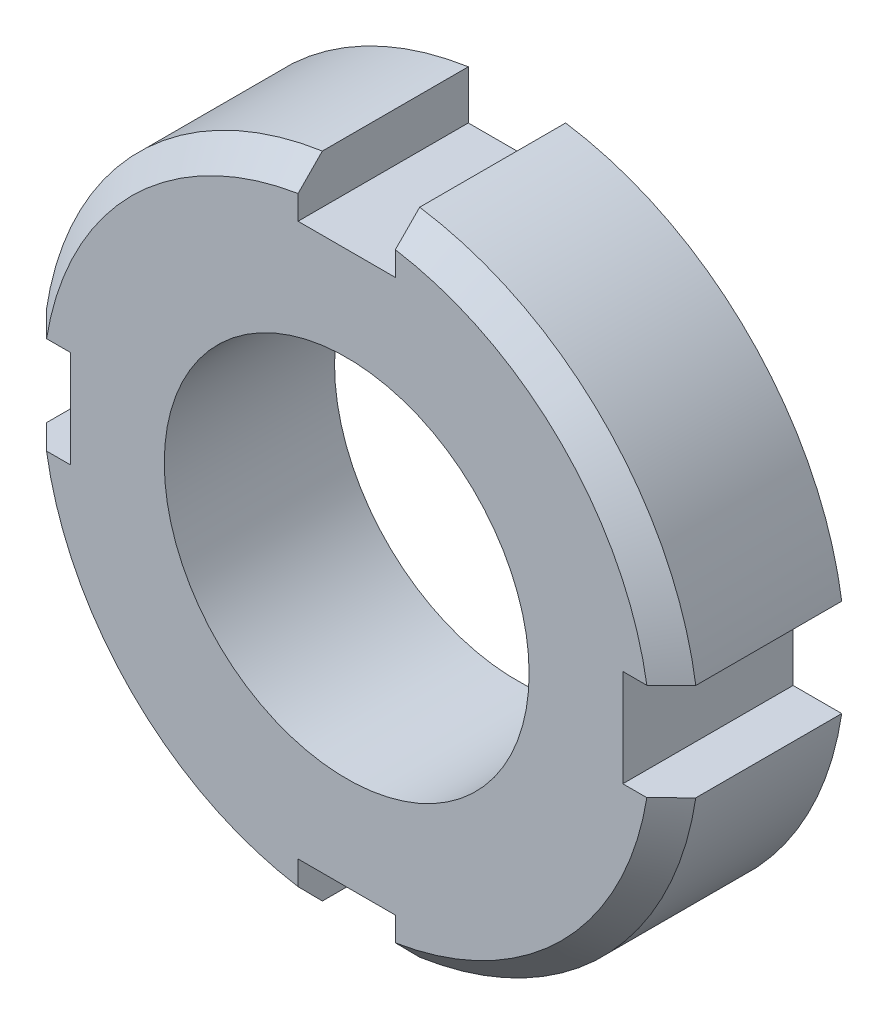
ISO-10303-21;
HEADER;
FILE_DESCRIPTION(('STEP AP214'),'2;1');
FILE_NAME('part.step','',(''),(''),'','','');
FILE_SCHEMA(('AUTOMOTIVE_DESIGN { 1 0 10303 214 1 1 1 1 }'));
ENDSEC;
DATA;
#1=APPLICATION_CONTEXT('core data for automotive mechanical design processes');
#2=APPLICATION_PROTOCOL_DEFINITION('international standard','automotive_design',2000,#1);
#3=PRODUCT_CONTEXT('',#1,'mechanical');
#4=PRODUCT('Part','Part','',(#3));
#5=PRODUCT_RELATED_PRODUCT_CATEGORY('part','',(#4));
#6=PRODUCT_DEFINITION_FORMATION('','',#4);
#7=PRODUCT_DEFINITION_CONTEXT('part definition',#1,'design');
#8=PRODUCT_DEFINITION('design','',#6,#7);
#9=PRODUCT_DEFINITION_SHAPE('','',#8);
#10=(LENGTH_UNIT() NAMED_UNIT(*) SI_UNIT(.MILLI.,.METRE.));
#11=(NAMED_UNIT(*) PLANE_ANGLE_UNIT() SI_UNIT($,.RADIAN.));
#12=(NAMED_UNIT(*) SI_UNIT($,.STERADIAN.) SOLID_ANGLE_UNIT());
#13=UNCERTAINTY_MEASURE_WITH_UNIT(LENGTH_MEASURE(1.E-05),#10,'distance_accuracy_value','');
#14=(GEOMETRIC_REPRESENTATION_CONTEXT(3) GLOBAL_UNCERTAINTY_ASSIGNED_CONTEXT((#13)) GLOBAL_UNIT_ASSIGNED_CONTEXT((#10,
#11,#12)) REPRESENTATION_CONTEXT('',''));
#15=CARTESIAN_POINT('',(0.,0.,0.));
#16=DIRECTION('',(0.,0.,1.));
#17=DIRECTION('',(1.,0.,0.));
#18=AXIS2_PLACEMENT_3D('',#15,#16,#17);
#19=CARTESIAN_POINT('',(-2.,11.3510299228187,3.5));
#20=DIRECTION('',(0.,-1.,0.));
#21=DIRECTION('',(0.,0.,-1.));
#22=AXIS2_PLACEMENT_3D('',#19,#20,#21);
#23=PLANE('',#22);
#24=DIRECTION('',(-1.,0.,0.));
#25=VECTOR('',#24,1.);
#26=CARTESIAN_POINT('',(-2.,11.3510299228187,-3.5));
#27=LINE('',#26,#25);
#28=CARTESIAN_POINT('',(2.,11.3510299228187,-3.5));
#29=VERTEX_POINT('',#28);
#30=CARTESIAN_POINT('',(-2.,11.3510299228187,-3.5));
#31=VERTEX_POINT('',#30);
#32=EDGE_CURVE('E211',#29,#31,#27,.T.);
#33=ORIENTED_EDGE('',*,*,#32,.T.);
#34=DIRECTION('',(0.,0.,-1.));
#35=VECTOR('',#34,1.);
#36=CARTESIAN_POINT('',(-2.,11.3510299228187,3.5));
#37=LINE('',#36,#35);
#38=CARTESIAN_POINT('',(-2.,11.3510299228187,3.5));
#39=VERTEX_POINT('',#38);
#40=EDGE_CURVE('E194',#39,#31,#37,.T.);
#41=ORIENTED_EDGE('',*,*,#40,.F.);
#42=DIRECTION('',(-1.,0.,0.));
#43=VECTOR('',#42,1.);
#44=CARTESIAN_POINT('',(-2.,11.3510299228187,3.5));
#45=LINE('',#44,#43);
#46=CARTESIAN_POINT('',(2.,11.3510299228187,3.5));
#47=VERTEX_POINT('',#46);
#48=EDGE_CURVE('E201',#47,#39,#45,.T.);
#49=ORIENTED_EDGE('',*,*,#48,.F.);
#50=DIRECTION('',(0.,0.,-1.));
#51=VECTOR('',#50,1.);
#52=CARTESIAN_POINT('',(2.,11.3510299228187,3.5));
#53=LINE('',#52,#51);
#54=EDGE_CURVE('E526',#47,#29,#53,.T.);
#55=ORIENTED_EDGE('',*,*,#54,.T.);
#56=EDGE_LOOP('',(#33,#41,#49,#55));
#57=FACE_BOUND('',#56,.T.);
#58=ADVANCED_FACE('F44',(#57),#23,.F.);
#59=CARTESIAN_POINT('',(-2.,11.3510299228187,3.5));
#60=DIRECTION('',(-1.,0.,0.));
#61=DIRECTION('',(0.,-1.,0.));
#62=AXIS2_PLACEMENT_3D('',#59,#60,#61);
#63=PLANE('',#62);
#64=DIRECTION('',(0.,0.,-1.));
#65=VECTOR('',#64,1.);
#66=CARTESIAN_POINT('',(-2.,13.3510299228187,3.5));
#67=LINE('',#66,#65);
#68=CARTESIAN_POINT('',(-2.,13.3510299228187,2.49999999999998));
#69=VERTEX_POINT('',#68);
#70=CARTESIAN_POINT('',(-2.,13.3510299228187,-3.5));
#71=VERTEX_POINT('',#70);
#72=EDGE_CURVE('E218',#69,#71,#67,.T.);
#73=ORIENTED_EDGE('',*,*,#72,.F.);
#74=CARTESIAN_POINT('',(-2.,13.3510299228187,2.49999999999998));
#75=CARTESIAN_POINT('',(-2.,13.1824298645057,2.66674542059407));
#76=CARTESIAN_POINT('',(-2.,13.0137908985623,2.83345146404985));
#77=CARTESIAN_POINT('',(-2.,12.6764351507074,3.16678479738352));
#78=CARTESIAN_POINT('',(-2.,12.5077183687956,3.33341208726107));
#79=CARTESIAN_POINT('',(-2.,12.3389626792531,3.5));
#80=B_SPLINE_CURVE_WITH_KNOTS('',3,(#74,#75,#76,#77,#78,#79),.UNSPECIFIED.,.F.,.F.,(4,2,4),(0.,
0.711386007616392,1.42277201821502),.UNSPECIFIED.);
#81=CARTESIAN_POINT('',(-2.,12.3389626792531,3.5));
#82=VERTEX_POINT('',#81);
#83=EDGE_CURVE('E198',#69,#82,#80,.T.);
#84=ORIENTED_EDGE('',*,*,#83,.T.);
#85=DIRECTION('',(0.,1.,0.));
#86=VECTOR('',#85,1.);
#87=CARTESIAN_POINT('',(-2.,11.3510299228187,3.5));
#88=LINE('',#87,#86);
#89=EDGE_CURVE('E190',#39,#82,#88,.T.);
#90=ORIENTED_EDGE('',*,*,#89,.F.);
#91=ORIENTED_EDGE('',*,*,#40,.T.);
#92=DIRECTION('',(0.,1.,0.));
#93=VECTOR('',#92,1.);
#94=CARTESIAN_POINT('',(-2.,11.3510299228187,-3.5));
#95=LINE('',#94,#93);
#96=EDGE_CURVE('E531',#31,#71,#95,.T.);
#97=ORIENTED_EDGE('',*,*,#96,.T.);
#98=EDGE_LOOP('',(#73,#84,#90,#91,#97));
#99=FACE_BOUND('',#98,.T.);
#100=ADVANCED_FACE('F188',(#99),#63,.F.);
#101=CARTESIAN_POINT('',(0.,0.,3.5));
#102=DIRECTION('',(0.,0.,-1.));
#103=DIRECTION('',(-1.,0.,0.));
#104=AXIS2_PLACEMENT_3D('',#101,#102,#103);
#105=CYLINDRICAL_SURFACE('',#104,13.5);
#106=DIRECTION('',(0.,0.,-1.));
#107=VECTOR('',#106,1.);
#108=CARTESIAN_POINT('',(-13.3510299228187,2.,3.5));
#109=LINE('',#108,#107);
#110=CARTESIAN_POINT('',(-13.3510299228187,2.,2.49999999999998));
#111=VERTEX_POINT('',#110);
#112=CARTESIAN_POINT('',(-13.3510299228187,2.,-3.5));
#113=VERTEX_POINT('',#112);
#114=EDGE_CURVE('E216',#111,#113,#109,.T.);
#115=ORIENTED_EDGE('',*,*,#114,.F.);
#116=CARTESIAN_POINT('',(0.,0.,2.49999999999998));
#117=DIRECTION('',(0.,0.,1.));
#118=DIRECTION('',(1.,0.,0.));
#119=AXIS2_PLACEMENT_3D('',#116,#117,#118);
#120=CIRCLE('',#119,13.5);
#121=EDGE_CURVE('E307',#111,#69,#120,.F.);
#122=ORIENTED_EDGE('',*,*,#121,.T.);
#123=ORIENTED_EDGE('',*,*,#72,.T.);
#124=CARTESIAN_POINT('',(0.,0.,-3.5));
#125=DIRECTION('',(0.,0.,1.));
#126=DIRECTION('',(1.,0.,0.));
#127=AXIS2_PLACEMENT_3D('',#124,#125,#126);
#128=CIRCLE('',#127,13.5);
#129=EDGE_CURVE('E537',#71,#113,#128,.T.);
#130=ORIENTED_EDGE('',*,*,#129,.T.);
#131=EDGE_LOOP('',(#115,#122,#123,#130));
#132=FACE_BOUND('',#131,.T.);
#133=ADVANCED_FACE('F319',(#132),#105,.T.);
#134=CARTESIAN_POINT('',(-11.3510299228187,2.,3.5));
#135=DIRECTION('',(0.,1.,0.));
#136=DIRECTION('',(-1.,0.,0.));
#137=AXIS2_PLACEMENT_3D('',#134,#135,#136);
#138=PLANE('',#137);
#139=DIRECTION('',(1.,0.,0.));
#140=VECTOR('',#139,1.);
#141=CARTESIAN_POINT('',(-11.3510299228187,2.,3.5));
#142=LINE('',#141,#140);
#143=CARTESIAN_POINT('',(-12.3389626792531,2.,3.5));
#144=VERTEX_POINT('',#143);
#145=CARTESIAN_POINT('',(-11.3510299228187,2.,3.5));
#146=VERTEX_POINT('',#145);
#147=EDGE_CURVE('E196',#144,#146,#142,.T.);
#148=ORIENTED_EDGE('',*,*,#147,.F.);
#149=CARTESIAN_POINT('',(-12.3389626792531,2.,3.5));
#150=CARTESIAN_POINT('',(-12.5077183687956,2.,3.33341208726107));
#151=CARTESIAN_POINT('',(-12.6764351507074,2.,3.16678479738352));
#152=CARTESIAN_POINT('',(-13.0137908985623,2.,2.83345146404985));
#153=CARTESIAN_POINT('',(-13.1824298645057,2.,2.66674542059407));
#154=CARTESIAN_POINT('',(-13.3510299228187,2.,2.49999999999998));
#155=B_SPLINE_CURVE_WITH_KNOTS('',3,(#149,#150,#151,#152,#153,#154),.UNSPECIFIED.,.F.,.F.,(4,2,
4),(0.,0.711386010598626,1.42277201821502),.UNSPECIFIED.);
#156=EDGE_CURVE('E303',#144,#111,#155,.T.);
#157=ORIENTED_EDGE('',*,*,#156,.T.);
#158=ORIENTED_EDGE('',*,*,#114,.T.);
#159=DIRECTION('',(1.,0.,0.));
#160=VECTOR('',#159,1.);
#161=CARTESIAN_POINT('',(-11.3510299228187,2.,-3.5));
#162=LINE('',#161,#160);
#163=CARTESIAN_POINT('',(-11.3510299228187,2.,-3.5));
#164=VERTEX_POINT('',#163);
#165=EDGE_CURVE('E536',#113,#164,#162,.T.);
#166=ORIENTED_EDGE('',*,*,#165,.T.);
#167=DIRECTION('',(0.,0.,-1.));
#168=VECTOR('',#167,1.);
#169=CARTESIAN_POINT('',(-11.3510299228187,2.,3.5));
#170=LINE('',#169,#168);
#171=EDGE_CURVE('E594',#146,#164,#170,.T.);
#172=ORIENTED_EDGE('',*,*,#171,.F.);
#173=EDGE_LOOP('',(#148,#157,#158,#166,#172));
#174=FACE_BOUND('',#173,.T.);
#175=ADVANCED_FACE('F313',(#174),#138,.F.);
#176=CARTESIAN_POINT('',(-11.3510299228187,-2.,3.5));
#177=DIRECTION('',(1.,0.,0.));
#178=DIRECTION('',(0.,0.,-1.));
#179=AXIS2_PLACEMENT_3D('',#176,#177,#178);
#180=PLANE('',#179);
#181=DIRECTION('',(0.,-1.,0.));
#182=VECTOR('',#181,1.);
#183=CARTESIAN_POINT('',(-11.3510299228187,-2.,-3.5));
#184=LINE('',#183,#182);
#185=CARTESIAN_POINT('',(-11.3510299228187,-2.,-3.5));
#186=VERTEX_POINT('',#185);
#187=EDGE_CURVE('E543',#164,#186,#184,.T.);
#188=ORIENTED_EDGE('',*,*,#187,.T.);
#189=DIRECTION('',(0.,0.,-1.));
#190=VECTOR('',#189,1.);
#191=CARTESIAN_POINT('',(-11.3510299228187,-2.,3.5));
#192=LINE('',#191,#190);
#193=CARTESIAN_POINT('',(-11.3510299228187,-2.,3.5));
#194=VERTEX_POINT('',#193);
#195=EDGE_CURVE('E595',#194,#186,#192,.T.);
#196=ORIENTED_EDGE('',*,*,#195,.F.);
#197=DIRECTION('',(0.,-1.,0.));
#198=VECTOR('',#197,1.);
#199=CARTESIAN_POINT('',(-11.3510299228187,-2.,3.5));
#200=LINE('',#199,#198);
#201=EDGE_CURVE('E618',#146,#194,#200,.T.);
#202=ORIENTED_EDGE('',*,*,#201,.F.);
#203=ORIENTED_EDGE('',*,*,#171,.T.);
#204=EDGE_LOOP('',(#188,#196,#202,#203));
#205=FACE_BOUND('',#204,.T.);
#206=ADVANCED_FACE('F295',(#205),#180,.F.);
#207=CARTESIAN_POINT('',(-11.3510299228187,-2.,3.5));
#208=DIRECTION('',(0.,-1.,0.));
#209=DIRECTION('',(1.,0.,0.));
#210=AXIS2_PLACEMENT_3D('',#207,#208,#209);
#211=PLANE('',#210);
#212=DIRECTION('',(0.,0.,-1.));
#213=VECTOR('',#212,1.);
#214=CARTESIAN_POINT('',(-13.3510299228187,-2.,3.5));
#215=LINE('',#214,#213);
#216=CARTESIAN_POINT('',(-13.3510299228187,-2.,2.5));
#217=VERTEX_POINT('',#216);
#218=CARTESIAN_POINT('',(-13.3510299228187,-2.,-3.5));
#219=VERTEX_POINT('',#218);
#220=EDGE_CURVE('E586',#217,#219,#215,.T.);
#221=ORIENTED_EDGE('',*,*,#220,.F.);
#222=CARTESIAN_POINT('',(-13.3510299228187,-2.,2.5));
#223=CARTESIAN_POINT('',(-13.1824298645057,-2.,2.66674542059408));
#224=CARTESIAN_POINT('',(-13.0137908985623,-2.,2.83345146404986));
#225=CARTESIAN_POINT('',(-12.6764351507074,-2.,3.16678479738353));
#226=CARTESIAN_POINT('',(-12.5077183687956,-2.,3.33341208726108));
#227=CARTESIAN_POINT('',(-12.3389626792531,-2.,3.5));
#228=B_SPLINE_CURVE_WITH_KNOTS('',3,(#222,#223,#224,#225,#226,#227),.UNSPECIFIED.,.F.,.F.,(4,2,
4),(0.,0.71138600761638,1.422772018215),.UNSPECIFIED.);
#229=CARTESIAN_POINT('',(-12.3389626792531,-2.,3.5));
#230=VERTEX_POINT('',#229);
#231=EDGE_CURVE('E300',#217,#230,#228,.T.);
#232=ORIENTED_EDGE('',*,*,#231,.T.);
#233=DIRECTION('',(-1.,0.,0.));
#234=VECTOR('',#233,1.);
#235=CARTESIAN_POINT('',(-11.3510299228187,-2.,3.5));
#236=LINE('',#235,#234);
#237=EDGE_CURVE('E615',#194,#230,#236,.T.);
#238=ORIENTED_EDGE('',*,*,#237,.F.);
#239=ORIENTED_EDGE('',*,*,#195,.T.);
#240=DIRECTION('',(-1.,0.,0.));
#241=VECTOR('',#240,1.);
#242=CARTESIAN_POINT('',(-11.3510299228187,-2.,-3.5));
#243=LINE('',#242,#241);
#244=EDGE_CURVE('E542',#186,#219,#243,.T.);
#245=ORIENTED_EDGE('',*,*,#244,.T.);
#246=EDGE_LOOP('',(#221,#232,#238,#239,#245));
#247=FACE_BOUND('',#246,.T.);
#248=ADVANCED_FACE('F288',(#247),#211,.F.);
#249=CARTESIAN_POINT('',(0.,0.,3.5));
#250=DIRECTION('',(0.,0.,-1.));
#251=DIRECTION('',(-1.,0.,0.));
#252=AXIS2_PLACEMENT_3D('',#249,#250,#251);
#253=CYLINDRICAL_SURFACE('',#252,13.5);
#254=DIRECTION('',(0.,0.,-1.));
#255=VECTOR('',#254,1.);
#256=CARTESIAN_POINT('',(-2.,-13.3510299228187,3.5));
#257=LINE('',#256,#255);
#258=CARTESIAN_POINT('',(-2.,-13.3510299228187,2.5));
#259=VERTEX_POINT('',#258);
#260=CARTESIAN_POINT('',(-2.,-13.3510299228187,-3.5));
#261=VERTEX_POINT('',#260);
#262=EDGE_CURVE('E587',#259,#261,#257,.T.);
#263=ORIENTED_EDGE('',*,*,#262,.F.);
#264=CARTESIAN_POINT('',(0.,0.,2.5));
#265=DIRECTION('',(0.,0.,1.));
#266=DIRECTION('',(1.,0.,0.));
#267=AXIS2_PLACEMENT_3D('',#264,#265,#266);
#268=CIRCLE('',#267,13.5);
#269=EDGE_CURVE('E277',#259,#217,#268,.F.);
#270=ORIENTED_EDGE('',*,*,#269,.T.);
#271=ORIENTED_EDGE('',*,*,#220,.T.);
#272=CARTESIAN_POINT('',(0.,0.,-3.5));
#273=DIRECTION('',(0.,0.,1.));
#274=DIRECTION('',(1.,0.,0.));
#275=AXIS2_PLACEMENT_3D('',#272,#273,#274);
#276=CIRCLE('',#275,13.5);
#277=EDGE_CURVE('E546',#219,#261,#276,.T.);
#278=ORIENTED_EDGE('',*,*,#277,.T.);
#279=EDGE_LOOP('',(#263,#270,#271,#278));
#280=FACE_BOUND('',#279,.T.);
#281=ADVANCED_FACE('F281',(#280),#253,.T.);
#282=CARTESIAN_POINT('',(-2.,-11.3510299228187,3.5));
#283=DIRECTION('',(-1.,0.,0.));
#284=DIRECTION('',(0.,-1.,0.));
#285=AXIS2_PLACEMENT_3D('',#282,#283,#284);
#286=PLANE('',#285);
#287=DIRECTION('',(0.,1.,0.));
#288=VECTOR('',#287,1.);
#289=CARTESIAN_POINT('',(-2.,-11.3510299228187,3.5));
#290=LINE('',#289,#288);
#291=CARTESIAN_POINT('',(-2.,-12.3389626792531,3.5));
#292=VERTEX_POINT('',#291);
#293=CARTESIAN_POINT('',(-2.,-11.3510299228187,3.5));
#294=VERTEX_POINT('',#293);
#295=EDGE_CURVE('E614',#292,#294,#290,.T.);
#296=ORIENTED_EDGE('',*,*,#295,.F.);
#297=CARTESIAN_POINT('',(-2.,-12.3389626792531,3.5));
#298=CARTESIAN_POINT('',(-2.,-12.5077183687956,3.33341208726108));
#299=CARTESIAN_POINT('',(-2.,-12.6764351507074,3.16678479738353));
#300=CARTESIAN_POINT('',(-2.,-13.0137908985623,2.83345146404986));
#301=CARTESIAN_POINT('',(-2.,-13.1824298645057,2.66674542059408));
#302=CARTESIAN_POINT('',(-2.,-13.3510299228187,2.5));
#303=B_SPLINE_CURVE_WITH_KNOTS('',3,(#297,#298,#299,#300,#301,#302),.UNSPECIFIED.,.F.,.F.,(4,2,
4),(0.,0.711386010598615,1.422772018215),.UNSPECIFIED.);
#304=EDGE_CURVE('E269',#292,#259,#303,.T.);
#305=ORIENTED_EDGE('',*,*,#304,.T.);
#306=ORIENTED_EDGE('',*,*,#262,.T.);
#307=DIRECTION('',(0.,1.,0.));
#308=VECTOR('',#307,1.);
#309=CARTESIAN_POINT('',(-2.,-11.3510299228187,-3.5));
#310=LINE('',#309,#308);
#311=CARTESIAN_POINT('',(-2.,-11.3510299228187,-3.5));
#312=VERTEX_POINT('',#311);
#313=EDGE_CURVE('E548',#261,#312,#310,.T.);
#314=ORIENTED_EDGE('',*,*,#313,.T.);
#315=DIRECTION('',(0.,0.,-1.));
#316=VECTOR('',#315,1.);
#317=CARTESIAN_POINT('',(-2.,-11.3510299228187,3.5));
#318=LINE('',#317,#316);
#319=EDGE_CURVE('E583',#294,#312,#318,.T.);
#320=ORIENTED_EDGE('',*,*,#319,.F.);
#321=EDGE_LOOP('',(#296,#305,#306,#314,#320));
#322=FACE_BOUND('',#321,.T.);
#323=ADVANCED_FACE('F283',(#322),#286,.F.);
#324=CARTESIAN_POINT('',(2.,-11.3510299228187,3.5));
#325=DIRECTION('',(0.,1.,0.));
#326=DIRECTION('',(0.,0.,1.));
#327=AXIS2_PLACEMENT_3D('',#324,#325,#326);
#328=PLANE('',#327);
#329=DIRECTION('',(1.,0.,0.));
#330=VECTOR('',#329,1.);
#331=CARTESIAN_POINT('',(2.,-11.3510299228187,-3.5));
#332=LINE('',#331,#330);
#333=CARTESIAN_POINT('',(2.,-11.3510299228187,-3.5));
#334=VERTEX_POINT('',#333);
#335=EDGE_CURVE('E553',#312,#334,#332,.T.);
#336=ORIENTED_EDGE('',*,*,#335,.T.);
#337=DIRECTION('',(0.,0.,-1.));
#338=VECTOR('',#337,1.);
#339=CARTESIAN_POINT('',(2.,-11.3510299228187,3.5));
#340=LINE('',#339,#338);
#341=CARTESIAN_POINT('',(2.,-11.3510299228187,3.5));
#342=VERTEX_POINT('',#341);
#343=EDGE_CURVE('E585',#342,#334,#340,.T.);
#344=ORIENTED_EDGE('',*,*,#343,.F.);
#345=DIRECTION('',(1.,0.,0.));
#346=VECTOR('',#345,1.);
#347=CARTESIAN_POINT('',(2.,-11.3510299228187,3.5));
#348=LINE('',#347,#346);
#349=EDGE_CURVE('E616',#294,#342,#348,.T.);
#350=ORIENTED_EDGE('',*,*,#349,.F.);
#351=ORIENTED_EDGE('',*,*,#319,.T.);
#352=EDGE_LOOP('',(#336,#344,#350,#351));
#353=FACE_BOUND('',#352,.T.);
#354=ADVANCED_FACE('F263',(#353),#328,.F.);
#355=CARTESIAN_POINT('',(2.,-11.3510299228187,3.5));
#356=DIRECTION('',(1.,0.,0.));
#357=DIRECTION('',(0.,1.,0.));
#358=AXIS2_PLACEMENT_3D('',#355,#356,#357);
#359=PLANE('',#358);
#360=DIRECTION('',(0.,0.,-1.));
#361=VECTOR('',#360,1.);
#362=CARTESIAN_POINT('',(2.,-13.3510299228187,3.5));
#363=LINE('',#362,#361);
#364=CARTESIAN_POINT('',(2.,-13.3510299228187,2.49999999999999));
#365=VERTEX_POINT('',#364);
#366=CARTESIAN_POINT('',(2.,-13.3510299228187,-3.5));
#367=VERTEX_POINT('',#366);
#368=EDGE_CURVE('E578',#365,#367,#363,.T.);
#369=ORIENTED_EDGE('',*,*,#368,.F.);
#370=CARTESIAN_POINT('',(2.,-13.3510299228187,2.49999999999999));
#371=CARTESIAN_POINT('',(2.,-13.1824298645057,2.66674542059407));
#372=CARTESIAN_POINT('',(2.,-13.0137908985623,2.83345146404985));
#373=CARTESIAN_POINT('',(2.,-12.6764351507074,3.16678479738352));
#374=CARTESIAN_POINT('',(2.,-12.5077183687956,3.33341208726107));
#375=CARTESIAN_POINT('',(2.,-12.3389626792531,3.5));
#376=B_SPLINE_CURVE_WITH_KNOTS('',3,(#370,#371,#372,#373,#374,#375),.UNSPECIFIED.,.F.,.F.,(4,2,
4),(0.,0.71138600761639,1.42277201821501),.UNSPECIFIED.);
#377=CARTESIAN_POINT('',(2.,-12.3389626792531,3.5));
#378=VERTEX_POINT('',#377);
#379=EDGE_CURVE('E265',#365,#378,#376,.T.);
#380=ORIENTED_EDGE('',*,*,#379,.T.);
#381=DIRECTION('',(0.,-1.,0.));
#382=VECTOR('',#381,1.);
#383=CARTESIAN_POINT('',(2.,-11.3510299228187,3.5));
#384=LINE('',#383,#382);
#385=EDGE_CURVE('E624',#342,#378,#384,.T.);
#386=ORIENTED_EDGE('',*,*,#385,.F.);
#387=ORIENTED_EDGE('',*,*,#343,.T.);
#388=DIRECTION('',(0.,-1.,0.));
#389=VECTOR('',#388,1.);
#390=CARTESIAN_POINT('',(2.,-11.3510299228187,-3.5));
#391=LINE('',#390,#389);
#392=EDGE_CURVE('E551',#334,#367,#391,.T.);
#393=ORIENTED_EDGE('',*,*,#392,.T.);
#394=EDGE_LOOP('',(#369,#380,#386,#387,#393));
#395=FACE_BOUND('',#394,.T.);
#396=ADVANCED_FACE('F257',(#395),#359,.F.);
#397=CARTESIAN_POINT('',(0.,0.,3.5));
#398=DIRECTION('',(0.,0.,-1.));
#399=DIRECTION('',(-1.,0.,0.));
#400=AXIS2_PLACEMENT_3D('',#397,#398,#399);
#401=CYLINDRICAL_SURFACE('',#400,13.5);
#402=DIRECTION('',(0.,0.,-1.));
#403=VECTOR('',#402,1.);
#404=CARTESIAN_POINT('',(13.3510299228187,-2.,3.5));
#405=LINE('',#404,#403);
#406=CARTESIAN_POINT('',(13.3510299228187,-2.,2.49999999999999));
#407=VERTEX_POINT('',#406);
#408=CARTESIAN_POINT('',(13.3510299228187,-2.,-3.5));
#409=VERTEX_POINT('',#408);
#410=EDGE_CURVE('E579',#407,#409,#405,.T.);
#411=ORIENTED_EDGE('',*,*,#410,.F.);
#412=CARTESIAN_POINT('',(0.,0.,2.49999999999999));
#413=DIRECTION('',(0.,0.,1.));
#414=DIRECTION('',(1.,0.,0.));
#415=AXIS2_PLACEMENT_3D('',#412,#413,#414);
#416=CIRCLE('',#415,13.5);
#417=EDGE_CURVE('E237',#407,#365,#416,.F.);
#418=ORIENTED_EDGE('',*,*,#417,.T.);
#419=ORIENTED_EDGE('',*,*,#368,.T.);
#420=CARTESIAN_POINT('',(0.,0.,-3.5));
#421=DIRECTION('',(0.,0.,1.));
#422=DIRECTION('',(1.,0.,0.));
#423=AXIS2_PLACEMENT_3D('',#420,#421,#422);
#424=CIRCLE('',#423,13.5);
#425=EDGE_CURVE('E558',#367,#409,#424,.T.);
#426=ORIENTED_EDGE('',*,*,#425,.T.);
#427=EDGE_LOOP('',(#411,#418,#419,#426));
#428=FACE_BOUND('',#427,.T.);
#429=ADVANCED_FACE('F255',(#428),#401,.T.);
#430=CARTESIAN_POINT('',(11.3510299228187,-2.,3.5));
#431=DIRECTION('',(0.,-1.,0.));
#432=DIRECTION('',(0.,0.,-1.));
#433=AXIS2_PLACEMENT_3D('',#430,#431,#432);
#434=PLANE('',#433);
#435=DIRECTION('',(-1.,0.,0.));
#436=VECTOR('',#435,1.);
#437=CARTESIAN_POINT('',(11.3510299228187,-2.,3.5));
#438=LINE('',#437,#436);
#439=CARTESIAN_POINT('',(12.3389626792531,-2.,3.5));
#440=VERTEX_POINT('',#439);
#441=CARTESIAN_POINT('',(11.3510299228187,-2.,3.5));
#442=VERTEX_POINT('',#441);
#443=EDGE_CURVE('E527',#440,#442,#438,.T.);
#444=ORIENTED_EDGE('',*,*,#443,.F.);
#445=CARTESIAN_POINT('',(12.3389626792531,-2.,3.5));
#446=CARTESIAN_POINT('',(12.5077183687956,-2.,3.33341208726107));
#447=CARTESIAN_POINT('',(12.6764351507074,-2.,3.16678479738352));
#448=CARTESIAN_POINT('',(13.0137908985623,-2.,2.83345146404985));
#449=CARTESIAN_POINT('',(13.1824298645057,-2.,2.66674542059407));
#450=CARTESIAN_POINT('',(13.3510299228187,-2.,2.49999999999999));
#451=B_SPLINE_CURVE_WITH_KNOTS('',3,(#445,#446,#447,#448,#449,#450),.UNSPECIFIED.,.F.,.F.,(4,2,
4),(0.,0.711386010598626,1.42277201821501),.UNSPECIFIED.);
#452=EDGE_CURVE('E233',#440,#407,#451,.T.);
#453=ORIENTED_EDGE('',*,*,#452,.T.);
#454=ORIENTED_EDGE('',*,*,#410,.T.);
#455=DIRECTION('',(-1.,0.,0.));
#456=VECTOR('',#455,1.);
#457=CARTESIAN_POINT('',(11.3510299228187,-2.,-3.5));
#458=LINE('',#457,#456);
#459=CARTESIAN_POINT('',(11.3510299228187,-2.,-3.5));
#460=VERTEX_POINT('',#459);
#461=EDGE_CURVE('E559',#409,#460,#458,.T.);
#462=ORIENTED_EDGE('',*,*,#461,.T.);
#463=DIRECTION('',(0.,0.,-1.));
#464=VECTOR('',#463,1.);
#465=CARTESIAN_POINT('',(11.3510299228187,-2.,3.5));
#466=LINE('',#465,#464);
#467=EDGE_CURVE('E574',#442,#460,#466,.T.);
#468=ORIENTED_EDGE('',*,*,#467,.F.);
#469=EDGE_LOOP('',(#444,#453,#454,#462,#468));
#470=FACE_BOUND('',#469,.T.);
#471=ADVANCED_FACE('F246',(#470),#434,.F.);
#472=CARTESIAN_POINT('',(11.3510299228187,2.,3.5));
#473=DIRECTION('',(-1.,0.,0.));
#474=DIRECTION('',(0.,0.,1.));
#475=AXIS2_PLACEMENT_3D('',#472,#473,#474);
#476=PLANE('',#475);
#477=DIRECTION('',(0.,1.,0.));
#478=VECTOR('',#477,1.);
#479=CARTESIAN_POINT('',(11.3510299228187,2.,-3.5));
#480=LINE('',#479,#478);
#481=CARTESIAN_POINT('',(11.3510299228187,2.,-3.5));
#482=VERTEX_POINT('',#481);
#483=EDGE_CURVE('E561',#460,#482,#480,.T.);
#484=ORIENTED_EDGE('',*,*,#483,.T.);
#485=DIRECTION('',(0.,0.,-1.));
#486=VECTOR('',#485,1.);
#487=CARTESIAN_POINT('',(11.3510299228187,2.,3.5));
#488=LINE('',#487,#486);
#489=CARTESIAN_POINT('',(11.3510299228187,2.,3.5));
#490=VERTEX_POINT('',#489);
#491=EDGE_CURVE('E572',#490,#482,#488,.T.);
#492=ORIENTED_EDGE('',*,*,#491,.F.);
#493=DIRECTION('',(0.,1.,0.));
#494=VECTOR('',#493,1.);
#495=CARTESIAN_POINT('',(11.3510299228187,2.,3.5));
#496=LINE('',#495,#494);
#497=EDGE_CURVE('E522',#442,#490,#496,.T.);
#498=ORIENTED_EDGE('',*,*,#497,.F.);
#499=ORIENTED_EDGE('',*,*,#467,.T.);
#500=EDGE_LOOP('',(#484,#492,#498,#499));
#501=FACE_BOUND('',#500,.T.);
#502=ADVANCED_FACE('F252',(#501),#476,.F.);
#503=CARTESIAN_POINT('',(11.3510299228187,2.,3.5));
#504=DIRECTION('',(0.,1.,0.));
#505=DIRECTION('',(0.,0.,1.));
#506=AXIS2_PLACEMENT_3D('',#503,#504,#505);
#507=PLANE('',#506);
#508=DIRECTION('',(0.,0.,-1.));
#509=VECTOR('',#508,1.);
#510=CARTESIAN_POINT('',(13.3510299228187,2.,3.5));
#511=LINE('',#510,#509);
#512=CARTESIAN_POINT('',(13.3510299228187,2.,2.49999999999998));
#513=VERTEX_POINT('',#512);
#514=CARTESIAN_POINT('',(13.3510299228187,2.,-3.5));
#515=VERTEX_POINT('',#514);
#516=EDGE_CURVE('E523',#513,#515,#511,.T.);
#517=ORIENTED_EDGE('',*,*,#516,.F.);
#518=CARTESIAN_POINT('',(13.3510299228187,2.,2.49999999999998));
#519=CARTESIAN_POINT('',(13.1824298645057,2.,2.66674542059407));
#520=CARTESIAN_POINT('',(13.0137908985623,2.,2.83345146404985));
#521=CARTESIAN_POINT('',(12.6764351507074,2.,3.16678479738352));
#522=CARTESIAN_POINT('',(12.5077183687956,2.,3.33341208726107));
#523=CARTESIAN_POINT('',(12.3389626792531,2.,3.5));
#524=B_SPLINE_CURVE_WITH_KNOTS('',3,(#518,#519,#520,#521,#522,#523),.UNSPECIFIED.,.F.,.F.,(4,2,
4),(0.,0.711386007616392,1.42277201821502),.UNSPECIFIED.);
#525=CARTESIAN_POINT('',(12.3389626792531,2.,3.5));
#526=VERTEX_POINT('',#525);
#527=EDGE_CURVE('E11',#513,#526,#524,.T.);
#528=ORIENTED_EDGE('',*,*,#527,.T.);
#529=DIRECTION('',(1.,0.,0.));
#530=VECTOR('',#529,1.);
#531=CARTESIAN_POINT('',(11.3510299228187,2.,3.5));
#532=LINE('',#531,#530);
#533=EDGE_CURVE('E516',#490,#526,#532,.T.);
#534=ORIENTED_EDGE('',*,*,#533,.F.);
#535=ORIENTED_EDGE('',*,*,#491,.T.);
#536=DIRECTION('',(1.,0.,0.));
#537=VECTOR('',#536,1.);
#538=CARTESIAN_POINT('',(11.3510299228187,2.,-3.5));
#539=LINE('',#538,#537);
#540=EDGE_CURVE('E563',#482,#515,#539,.T.);
#541=ORIENTED_EDGE('',*,*,#540,.T.);
#542=EDGE_LOOP('',(#517,#528,#534,#535,#541));
#543=FACE_BOUND('',#542,.T.);
#544=ADVANCED_FACE('F341',(#543),#507,.F.);
#545=CARTESIAN_POINT('',(0.,0.,3.5));
#546=DIRECTION('',(0.,0.,-1.));
#547=DIRECTION('',(-1.,0.,0.));
#548=AXIS2_PLACEMENT_3D('',#545,#546,#547);
#549=CYLINDRICAL_SURFACE('',#548,13.5);
#550=DIRECTION('',(0.,0.,-1.));
#551=VECTOR('',#550,1.);
#552=CARTESIAN_POINT('',(2.,13.3510299228187,3.5));
#553=LINE('',#552,#551);
#554=CARTESIAN_POINT('',(2.,13.3510299228187,2.49999999999998));
#555=VERTEX_POINT('',#554);
#556=CARTESIAN_POINT('',(2.,13.3510299228187,-3.5));
#557=VERTEX_POINT('',#556);
#558=EDGE_CURVE('E569',#555,#557,#553,.T.);
#559=ORIENTED_EDGE('',*,*,#558,.F.);
#560=CARTESIAN_POINT('',(0.,0.,2.49999999999998));
#561=DIRECTION('',(0.,0.,1.));
#562=DIRECTION('',(1.,0.,0.));
#563=AXIS2_PLACEMENT_3D('',#560,#561,#562);
#564=CIRCLE('',#563,13.5);
#565=EDGE_CURVE('E58',#555,#513,#564,.F.);
#566=ORIENTED_EDGE('',*,*,#565,.T.);
#567=ORIENTED_EDGE('',*,*,#516,.T.);
#568=CARTESIAN_POINT('',(0.,0.,-3.5));
#569=DIRECTION('',(0.,0.,1.));
#570=DIRECTION('',(1.,0.,0.));
#571=AXIS2_PLACEMENT_3D('',#568,#569,#570);
#572=CIRCLE('',#571,13.5);
#573=EDGE_CURVE('E564',#515,#557,#572,.T.);
#574=ORIENTED_EDGE('',*,*,#573,.T.);
#575=EDGE_LOOP('',(#559,#566,#567,#574));
#576=FACE_BOUND('',#575,.T.);
#577=ADVANCED_FACE('F338',(#576),#549,.T.);
#578=CARTESIAN_POINT('',(2.,11.3510299228187,3.5));
#579=DIRECTION('',(1.,0.,0.));
#580=DIRECTION('',(0.,1.,0.));
#581=AXIS2_PLACEMENT_3D('',#578,#579,#580);
#582=PLANE('',#581);
#583=DIRECTION('',(0.,-1.,0.));
#584=VECTOR('',#583,1.);
#585=CARTESIAN_POINT('',(2.,11.3510299228187,3.5));
#586=LINE('',#585,#584);
#587=CARTESIAN_POINT('',(2.,12.3389626792531,3.5));
#588=VERTEX_POINT('',#587);
#589=EDGE_CURVE('E210',#588,#47,#586,.T.);
#590=ORIENTED_EDGE('',*,*,#589,.F.);
#591=CARTESIAN_POINT('',(2.,12.3389626792531,3.5));
#592=CARTESIAN_POINT('',(2.,12.5077183687956,3.33341208726107));
#593=CARTESIAN_POINT('',(2.,12.6764351507074,3.16678479738352));
#594=CARTESIAN_POINT('',(2.,13.0137908985623,2.83345146404985));
#595=CARTESIAN_POINT('',(2.,13.1824298645057,2.66674542059407));
#596=CARTESIAN_POINT('',(2.,13.3510299228187,2.49999999999998));
#597=B_SPLINE_CURVE_WITH_KNOTS('',3,(#591,#592,#593,#594,#595,#596),.UNSPECIFIED.,.F.,.F.,(4,2,
4),(0.,0.711386010598626,1.42277201821502),.UNSPECIFIED.);
#598=EDGE_CURVE('E73',#588,#555,#597,.T.);
#599=ORIENTED_EDGE('',*,*,#598,.T.);
#600=ORIENTED_EDGE('',*,*,#558,.T.);
#601=DIRECTION('',(0.,-1.,0.));
#602=VECTOR('',#601,1.);
#603=CARTESIAN_POINT('',(2.,11.3510299228187,-3.5));
#604=LINE('',#603,#602);
#605=EDGE_CURVE('E212',#557,#29,#604,.T.);
#606=ORIENTED_EDGE('',*,*,#605,.T.);
#607=ORIENTED_EDGE('',*,*,#54,.F.);
#608=EDGE_LOOP('',(#590,#599,#600,#606,#607));
#609=FACE_BOUND('',#608,.T.);
#610=ADVANCED_FACE('F334',(#609),#582,.F.);
#611=CARTESIAN_POINT('',(0.,0.,3.5));
#612=DIRECTION('',(0.,0.,1.));
#613=DIRECTION('',(1.,0.,0.));
#614=AXIS2_PLACEMENT_3D('',#611,#612,#613);
#615=PLANE('',#614);
#616=CARTESIAN_POINT('',(0.,0.,3.5));
#617=DIRECTION('',(0.,0.,1.));
#618=DIRECTION('',(1.,0.,0.));
#619=AXIS2_PLACEMENT_3D('',#616,#617,#618);
#620=CIRCLE('',#619,7.5);
#621=CARTESIAN_POINT('',(7.5,0.,3.5));
#622=VERTEX_POINT('',#621);
#623=EDGE_CURVE('E632',#622,#622,#620,.T.);
#624=ORIENTED_EDGE('',*,*,#623,.F.);
#625=EDGE_LOOP('',(#624));
#626=FACE_BOUND('',#625,.T.);
#627=ORIENTED_EDGE('',*,*,#385,.T.);
#628=CARTESIAN_POINT('',(0.,0.,3.5));
#629=DIRECTION('',(0.,0.,1.));
#630=DIRECTION('',(1.,0.,0.));
#631=AXIS2_PLACEMENT_3D('',#628,#629,#630);
#632=CIRCLE('',#631,12.5);
#633=EDGE_CURVE('E226',#378,#440,#632,.T.);
#634=ORIENTED_EDGE('',*,*,#633,.T.);
#635=ORIENTED_EDGE('',*,*,#443,.T.);
#636=ORIENTED_EDGE('',*,*,#497,.T.);
#637=ORIENTED_EDGE('',*,*,#533,.T.);
#638=CARTESIAN_POINT('',(0.,0.,3.5));
#639=DIRECTION('',(0.,0.,1.));
#640=DIRECTION('',(1.,0.,0.));
#641=AXIS2_PLACEMENT_3D('',#638,#639,#640);
#642=CIRCLE('',#641,12.5);
#643=EDGE_CURVE('E213',#526,#588,#642,.T.);
#644=ORIENTED_EDGE('',*,*,#643,.T.);
#645=ORIENTED_EDGE('',*,*,#589,.T.);
#646=ORIENTED_EDGE('',*,*,#48,.T.);
#647=ORIENTED_EDGE('',*,*,#89,.T.);
#648=CARTESIAN_POINT('',(0.,0.,3.5));
#649=DIRECTION('',(0.,0.,1.));
#650=DIRECTION('',(1.,0.,0.));
#651=AXIS2_PLACEMENT_3D('',#648,#649,#650);
#652=CIRCLE('',#651,12.5);
#653=EDGE_CURVE('E217',#82,#144,#652,.T.);
#654=ORIENTED_EDGE('',*,*,#653,.T.);
#655=ORIENTED_EDGE('',*,*,#147,.T.);
#656=ORIENTED_EDGE('',*,*,#201,.T.);
#657=ORIENTED_EDGE('',*,*,#237,.T.);
#658=CARTESIAN_POINT('',(0.,0.,3.5));
#659=DIRECTION('',(0.,0.,1.));
#660=DIRECTION('',(1.,0.,0.));
#661=AXIS2_PLACEMENT_3D('',#658,#659,#660);
#662=CIRCLE('',#661,12.5);
#663=EDGE_CURVE('E224',#230,#292,#662,.T.);
#664=ORIENTED_EDGE('',*,*,#663,.T.);
#665=ORIENTED_EDGE('',*,*,#295,.T.);
#666=ORIENTED_EDGE('',*,*,#349,.T.);
#667=EDGE_LOOP('',(#627,#634,#635,#636,#637,#644,#645,#646,#647,#654,#655,#656,#657,#664,#665,#666));
#668=FACE_BOUND('',#667,.T.);
#669=ADVANCED_FACE('F204',(#626,#668),#615,.T.);
#670=CARTESIAN_POINT('',(0.,0.,-3.5));
#671=DIRECTION('',(0.,0.,1.));
#672=DIRECTION('',(1.,0.,0.));
#673=AXIS2_PLACEMENT_3D('',#670,#671,#672);
#674=PLANE('',#673);
#675=CARTESIAN_POINT('',(0.,0.,-3.5));
#676=DIRECTION('',(0.,0.,1.));
#677=DIRECTION('',(1.,0.,0.));
#678=AXIS2_PLACEMENT_3D('',#675,#676,#677);
#679=CIRCLE('',#678,7.5);
#680=CARTESIAN_POINT('',(7.5,0.,-3.5));
#681=VERTEX_POINT('',#680);
#682=EDGE_CURVE('E534',#681,#681,#679,.T.);
#683=ORIENTED_EDGE('',*,*,#682,.T.);
#684=EDGE_LOOP('',(#683));
#685=FACE_BOUND('',#684,.T.);
#686=ORIENTED_EDGE('',*,*,#32,.F.);
#687=ORIENTED_EDGE('',*,*,#605,.F.);
#688=ORIENTED_EDGE('',*,*,#573,.F.);
#689=ORIENTED_EDGE('',*,*,#540,.F.);
#690=ORIENTED_EDGE('',*,*,#483,.F.);
#691=ORIENTED_EDGE('',*,*,#461,.F.);
#692=ORIENTED_EDGE('',*,*,#425,.F.);
#693=ORIENTED_EDGE('',*,*,#392,.F.);
#694=ORIENTED_EDGE('',*,*,#335,.F.);
#695=ORIENTED_EDGE('',*,*,#313,.F.);
#696=ORIENTED_EDGE('',*,*,#277,.F.);
#697=ORIENTED_EDGE('',*,*,#244,.F.);
#698=ORIENTED_EDGE('',*,*,#187,.F.);
#699=ORIENTED_EDGE('',*,*,#165,.F.);
#700=ORIENTED_EDGE('',*,*,#129,.F.);
#701=ORIENTED_EDGE('',*,*,#96,.F.);
#702=EDGE_LOOP('',(#686,#687,#688,#689,#690,#691,#692,#693,#694,#695,#696,#697,#698,#699,#700,#701));
#703=FACE_BOUND('',#702,.T.);
#704=ADVANCED_FACE('F342',(#685,#703),#674,.F.);
#705=CARTESIAN_POINT('',(0.,0.,-3.5));
#706=DIRECTION('',(0.,0.,1.));
#707=DIRECTION('',(1.,0.,0.));
#708=AXIS2_PLACEMENT_3D('',#705,#706,#707);
#709=CYLINDRICAL_SURFACE('',#708,7.5);
#710=ORIENTED_EDGE('',*,*,#682,.F.);
#711=EDGE_LOOP('',(#710));
#712=FACE_BOUND('',#711,.T.);
#713=ORIENTED_EDGE('',*,*,#623,.T.);
#714=EDGE_LOOP('',(#713));
#715=FACE_BOUND('',#714,.T.);
#716=ADVANCED_FACE('F389',(#712,#715),#709,.F.);
#717=CARTESIAN_POINT('',(0.,0.,3.5));
#718=DIRECTION('',(0.,0.,-1.));
#719=DIRECTION('',(-1.,0.,0.));
#720=AXIS2_PLACEMENT_3D('',#717,#718,#719);
#721=CONICAL_SURFACE('',#720,12.5,0.785398163397447);
#722=ORIENTED_EDGE('',*,*,#379,.F.);
#723=ORIENTED_EDGE('',*,*,#417,.F.);
#724=ORIENTED_EDGE('',*,*,#452,.F.);
#725=ORIENTED_EDGE('',*,*,#633,.F.);
#726=EDGE_LOOP('',(#722,#723,#724,#725));
#727=FACE_BOUND('',#726,.T.);
#728=ADVANCED_FACE('F245',(#727),#721,.T.);
#729=CARTESIAN_POINT('',(0.,0.,3.5));
#730=DIRECTION('',(0.,0.,-1.));
#731=DIRECTION('',(-1.,0.,0.));
#732=AXIS2_PLACEMENT_3D('',#729,#730,#731);
#733=CONICAL_SURFACE('',#732,12.5,0.785398163397449);
#734=ORIENTED_EDGE('',*,*,#231,.F.);
#735=ORIENTED_EDGE('',*,*,#269,.F.);
#736=ORIENTED_EDGE('',*,*,#304,.F.);
#737=ORIENTED_EDGE('',*,*,#663,.F.);
#738=EDGE_LOOP('',(#734,#735,#736,#737));
#739=FACE_BOUND('',#738,.T.);
#740=ADVANCED_FACE('F276',(#739),#733,.T.);
#741=CARTESIAN_POINT('',(0.,0.,3.5));
#742=DIRECTION('',(0.,0.,-1.));
#743=DIRECTION('',(-1.,0.,0.));
#744=AXIS2_PLACEMENT_3D('',#741,#742,#743);
#745=CONICAL_SURFACE('',#744,12.5,0.785398163397447);
#746=ORIENTED_EDGE('',*,*,#83,.F.);
#747=ORIENTED_EDGE('',*,*,#121,.F.);
#748=ORIENTED_EDGE('',*,*,#156,.F.);
#749=ORIENTED_EDGE('',*,*,#653,.F.);
#750=EDGE_LOOP('',(#746,#747,#748,#749));
#751=FACE_BOUND('',#750,.T.);
#752=ADVANCED_FACE('F315',(#751),#745,.T.);
#753=CARTESIAN_POINT('',(0.,0.,3.5));
#754=DIRECTION('',(0.,0.,-1.));
#755=DIRECTION('',(-1.,0.,0.));
#756=AXIS2_PLACEMENT_3D('',#753,#754,#755);
#757=CONICAL_SURFACE('',#756,12.5,0.785398163397447);
#758=ORIENTED_EDGE('',*,*,#527,.F.);
#759=ORIENTED_EDGE('',*,*,#565,.F.);
#760=ORIENTED_EDGE('',*,*,#598,.F.);
#761=ORIENTED_EDGE('',*,*,#643,.F.);
#762=EDGE_LOOP('',(#758,#759,#760,#761));
#763=FACE_BOUND('',#762,.T.);
#764=ADVANCED_FACE('F48',(#763),#757,.T.);
#765=CLOSED_SHELL('',(#58,#100,#133,#175,#206,#248,#281,#323,#354,#396,#429,#471,#502,#544,#577,
#610,#669,#704,#716,#728,#740,#752,#764));
#766=MANIFOLD_SOLID_BREP('B2',#765);
#767=ADVANCED_BREP_SHAPE_REPRESENTATION('',(#18,#766),#14);
#768=SHAPE_DEFINITION_REPRESENTATION(#9,#767);
ENDSEC;
END-ISO-10303-21;
